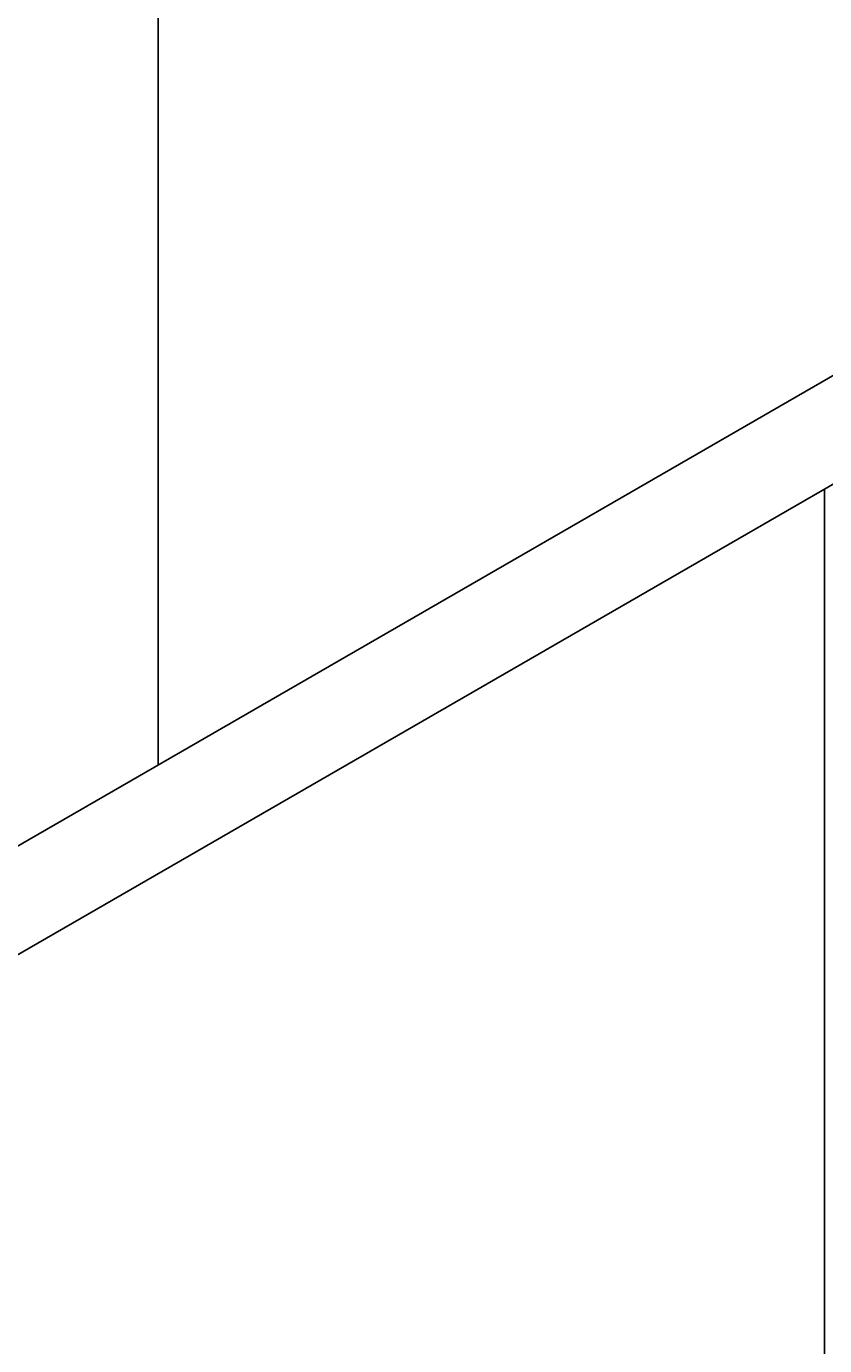
# Model space of a CAD drawing. Units: metres. Extents: x -2391 to 4922, y -635 to 4845.
# Tile 25 of 37: x 31 to 551, y 3127 to 3986. Entities that reach past the tile are written whole.
import ezdxf

# ---------------------------------------------------------------- set-up
doc = ezdxf.new("R2010")
doc.units = ezdxf.units.M
doc.header["$MEASUREMENT"] = 0
doc.layers.add('A-ANNO-DIMS', color=2, linetype='Continuous', lineweight=18)
doc.layers.add('A-FLOR-FIXT', color=3, linetype='Continuous', lineweight=25)
doc.styles.get("Standard").update_dxf_attribs({"font": 'arial.ttf'})
doc.dimstyles.get("Standard").update_dxf_attribs({"dimtxt": 5, "dimasz": 4, "dimexe": 0.18, "dimexo": 0.0625, "dimgap": 0.09, "dimtad": 0, "dimtih": 1, "dimtoh": 1, "dimdec": 0, "dimzin": 0, "dimdsep": 46, "dimtxsty": 'Standard', "dimcen": 0.09, "dimadec": 0, "dimazin": 0, "dimtfac": 1, "dimtdec": 0, "dimtofl": 0, "dimtmove": 0, "dimatfit": 3, "dimfxl": 1, "dimtolj": 1, "dimtzin": 0, "dimarcsym": 0})

# ---------------------------------------------------------------- blocks, each defined once
blk = doc.blocks.new('*D9')
at = {"layer": 'A-ANNO-DIMS', "color": 0, "lineweight": -2, "transparency": 16777216}
for p, q in [((-2047.33, 3005.34), (-2047.33, 4841.96)), ((-2043.33, 4841.78), (-755.9, 4841.78)), ((546.74, 4841.78), (-740.69, 4841.78)), ((550.74, 4505.34), (550.74, 4841.96))]:
    blk.add_line(p, q, dxfattribs=at)
at = {"layer": 'A-ANNO-DIMS', "color": 0, "transparency": 16777216}
for points in [[(-2043.33, 4842.44), (-2043.33, 4841.11), (-2047.33, 4841.78)], [(546.74, 4842.44), (546.74, 4841.11), (550.74, 4841.78)]]:
    blk.add_solid(points, dxfattribs=at)
at = {"layer": 'Defpoints', "color": 0, "transparency": 16777216}
for p in [(550.74, 4841.78), (550.74, 4505.28), (-2047.33, 3005.28)]:
    blk.add_point(p, dxfattribs=at)
at = {"layer": 'A-ANNO-DIMS', "color": 0, "transparency": 16777216, "insert": (-748.3, 4841.78), "char_height": 5, "attachment_point": 5}
blk.add_mtext('\\A1;2598', dxfattribs=at)
blk = doc.blocks.new('*D10')
at = {"layer": 'A-ANNO-DIMS', "color": 0, "lineweight": -2, "transparency": 16777216}
for p, q in [((550.68, 4505.28), (-2384.01, 4505.28)), ((-2383.83, 4501.28), (-2383.83, 2107.92)), ((-2383.83, -290.72), (-2383.83, 2102.63)), ((-488.55, -294.72), (-2384.01, -294.72))]:
    blk.add_line(p, q, dxfattribs=at)
at = {"layer": 'A-ANNO-DIMS', "color": 0, "transparency": 16777216}
for points in [[(-2384.5, 4501.28), (-2383.17, 4501.28), (-2383.83, 4505.28)], [(-2384.5, -290.72), (-2383.17, -290.72), (-2383.83, -294.72)]]:
    blk.add_solid(points, dxfattribs=at)
at = {"layer": 'Defpoints', "color": 0, "transparency": 16777216}
for p in [(-2383.83, 4505.28), (550.74, 4505.28), (-488.49, -294.72)]:
    blk.add_point(p, dxfattribs=at)
at = {"layer": 'A-ANNO-DIMS', "color": 0, "transparency": 16777216, "insert": (-2383.83, 2105.28), "char_height": 5, "attachment_point": 5}
blk.add_mtext('\\A1;4800', dxfattribs=at)

msp = doc.modelspace()

# ---------------------------------------------------------------- linework, layer by layer
at = {"layer": 'A-FLOR-FIXT'}
for p, q in [((116.9223, 3504.8104), (116.9223, 4254.8104)), ((612.0233, 3790.6571), (-878.2, 2930.2763)), ((612.0233, 3719.8954), (-816.9186, 2894.8954)), ((550.7419, 3005.2763), (550.7419, 3684.5146))]:
    msp.add_line(p, q, dxfattribs=at)

# ---------------------------------------------------------------- dimensions: what is measured, and where the dimension line sits
at = {"layer": 'A-ANNO-DIMS'}
dim = msp.add_linear_dim(base=(550.7419, 4841.7763), p1=(-2047.3343, 3005.2763), p2=(550.7419, 4505.2763), dimstyle='Standard', override={"dimdec": 0, "dimlfac": 1, "dimrnd": 0, "dimzin": 0, "dimdsep": 46, "dimlunit": 2}, dxfattribs=at)
dim.commit()
dim.dimension.update_dxf_attribs({"geometry": '*D9', "text_midpoint": (-748.2962, 4841.7763)})
dim = msp.add_linear_dim(base=(-2383.8343, 4505.2763), p1=(-488.4886, -294.7237), p2=(550.7419, 4505.2763), angle=90, dimstyle='Standard', override={"dimdec": 0, "dimlfac": 1, "dimrnd": 0, "dimzin": 0, "dimdsep": 46, "dimlunit": 2}, dxfattribs=at)
dim.commit()
dim.dimension.update_dxf_attribs({"geometry": '*D10', "text_midpoint": (-2383.8343, 2105.2763)})

doc.saveas('drawing.dxf')
